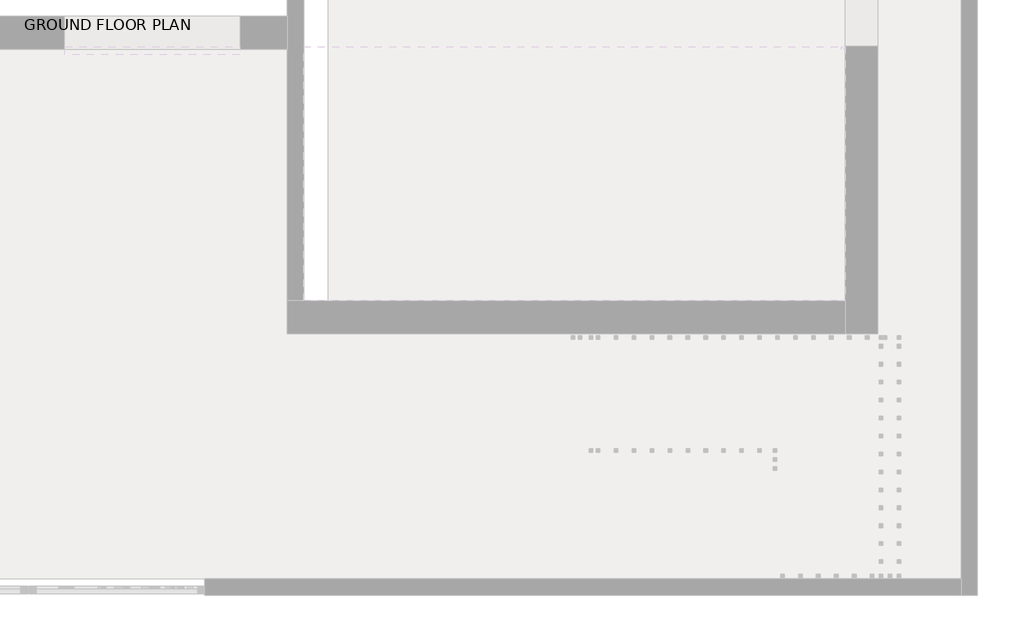
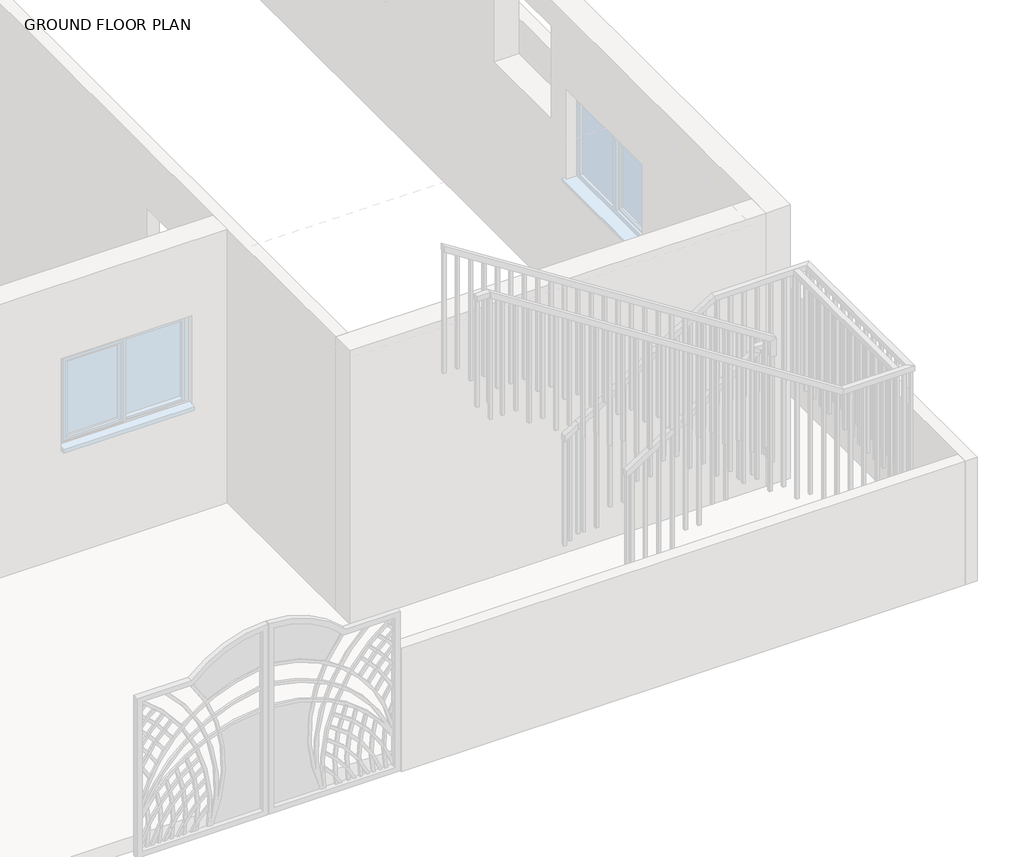
# One storey, part 20 of 23: 2 railings.
"""IFC4 building model written with IfcOpenShell, lengths in millimetres."""

from ifc_helpers import new_model, si_unit, frame, origin, place, context, project, spatial, polyline, outline, extrude, faceted_brep, element, save

model = new_model("IFC4")

# Units and contexts
model_context = context("Model", 3, world=origin())
ifc_project = project(units=[si_unit("LENGTHUNIT", "METRE", prefix="MILLI")], contexts=[model_context])

# Site, building, storey
site = spatial("IfcSite", under=ifc_project)
building = spatial("IfcBuilding", under=site)
storey = spatial("IfcBuildingStorey", under=building, Name="GROUND FLOOR PLAN", Elevation=487.68)

# Railings
placement = place(None, origin())
element("IfcRailing", 1, ObjectType="1100mm", at=placement, inside=storey, context=model_context, shape_type="SolidModel", body=[
    faceted_brep([(-8680.149573, -10220.0521308, 1912.8), (-8680.149573, -10220.0521308, 1853.4423995), (-8680.149573, -10270.0521308, 1853.4423995), (-8680.149573, -10270.0521308, 1912.8), (-7409.7306254, -10220.0521308, 2725.6), (-7395.1045513, -10220.0521308, 2675.6), (-7395.1045513, -10270.0521308, 2675.6), (-7409.7306254, -10270.0521308, 2725.6), (-6495.8132565, -10220.0521308, 2725.6), (-6495.8132565, -10220.0521308, 2675.6), (-6545.8132565, -10270.0521308, 2675.6), (-6545.8132565, -10270.0521308, 2725.6), (-6495.8132565, -11933.6860066, 2725.6), (-6495.8132565, -11933.6860066, 2675.6), (-6545.8132565, -11883.6860066, 2675.6), (-6545.8132565, -11883.6860066, 2725.6), (-7155.718398, -11933.6860066, 2725.6), (-7170.3479429, -11933.6860066, 2675.6), (-7170.3479429, -11883.6860066, 2675.6), (-7155.718398, -11883.6860066, 2725.6), (-10457.8773536, -11933.6860066, 4838.88), (-10457.8773536, -11883.6860066, 4838.88), (-10457.8773536, -11883.6860066, 4779.517542), (-10457.8773536, -11933.6860066, 4779.517542)], [[[0, 1, 2, 3]], [[1, 0, 4, 5]], [[2, 1, 5, 6]], [[3, 2, 6, 7]], [[0, 3, 7, 4]], [[5, 4, 8, 9]], [[6, 5, 9, 10]], [[7, 6, 10, 11]], [[4, 7, 11, 8]], [[9, 8, 12, 13]], [[10, 9, 13, 14]], [[11, 10, 14, 15]], [[8, 11, 15, 12]], [[13, 12, 16, 17]], [[14, 13, 17, 18]], [[15, 14, 18, 19]], [[12, 15, 19, 16]], [[20, 21, 22, 23]], [[17, 16, 20, 23]], [[18, 17, 23, 22]], [[19, 18, 22, 21]], [[16, 19, 21, 20]]]),
    extrude(outline(polyline([(4691.8007425, -10320.8132565), (4707.7999723, -10345.8132565), (3576.32, -10345.8132565), (3576.32, -10320.8132565), (4691.8007425, -10320.8132565)])), frame((0.0, -11921.1860066, 0.0), z_axis=(0.0, 1.0, 0.0), x_axis=(0.0, 0.0, 1.0)), (0.0, 0.0, 1.0), 25.0),
    extrude(outline(polyline([(4611.8045935, -10195.8132565), (4627.8038233, -10220.8132565), (3576.32, -10220.8132565), (3576.32, -10195.8132565), (4611.8045935, -10195.8132565)])), frame((0.0, -11921.1860066, 0.0), z_axis=(0.0, 1.0, 0.0), x_axis=(0.0, 0.0, 1.0)), (0.0, 0.0, 1.0), 25.0),
    extrude(outline(polyline([(4531.8084444, -10070.8132565), (4547.8076742, -10095.8132565), (3413.76, -10095.8132565), (3413.76, -10070.8132565), (4531.8084444, -10070.8132565)])), frame((0.0, -11921.1860066, 0.0), z_axis=(0.0, 1.0, 0.0), x_axis=(0.0, 0.0, 1.0)), (0.0, 0.0, 1.0), 25.0),
    extrude(outline(polyline([(4451.8122954, -9945.8132565), (4467.8115252, -9970.8132565), (3413.76, -9970.8132565), (3413.76, -9945.8132565), (4451.8122954, -9945.8132565)])), frame((0.0, -11921.1860066, 0.0), z_axis=(0.0, 1.0, 0.0), x_axis=(0.0, 0.0, 1.0)), (0.0, 0.0, 1.0), 25.0),
    extrude(outline(polyline([(4371.8161463, -9820.8132565), (4387.8153761, -9845.8132565), (3251.2, -9845.8132565), (3251.2, -9820.8132565), (4371.8161463, -9820.8132565)])), frame((0.0, -11921.1860066, 0.0), z_axis=(0.0, 1.0, 0.0), x_axis=(0.0, 0.0, 1.0)), (0.0, 0.0, 1.0), 25.0),
    extrude(outline(polyline([(4291.8423995, -9695.8132565), (4307.8371231, -9720.8132565), (3251.2, -9720.8132565), (3251.2, -9695.8132565), (4291.8423995, -9695.8132565)])), frame((0.0, -11921.1860066, 0.0), z_axis=(0.0, 1.0, 0.0), x_axis=(0.0, 0.0, 1.0)), (0.0, 0.0, 1.0), 25.0),
    extrude(outline(polyline([(4211.8238482, -9570.8132565), (4227.823078, -9595.8132565), (3088.64, -9595.8132565), (3088.64, -9570.8132565), (4211.8238482, -9570.8132565)])), frame((0.0, -11921.1860066, 0.0), z_axis=(0.0, 1.0, 0.0), x_axis=(0.0, 0.0, 1.0)), (0.0, 0.0, 1.0), 25.0),
    extrude(outline(polyline([(4131.8276992, -9445.8132565), (4147.826929, -9470.8132565), (3088.64, -9470.8132565), (3088.64, -9445.8132565), (4131.8276992, -9445.8132565)])), frame((0.0, -11921.1860066, 0.0), z_axis=(0.0, 1.0, 0.0), x_axis=(0.0, 0.0, 1.0)), (0.0, 0.0, 1.0), 25.0),
    extrude(outline(polyline([(4051.8315501, -9320.8132565), (4067.8307799, -9345.8132565), (2926.08, -9345.8132565), (2926.08, -9320.8132565), (4051.8315501, -9320.8132565)])), frame((0.0, -11921.1860066, 0.0), z_axis=(0.0, 1.0, 0.0), x_axis=(0.0, 0.0, 1.0)), (0.0, 0.0, 1.0), 25.0),
    extrude(outline(polyline([(3971.835401, -9195.8132565), (3987.8346309, -9220.8132565), (2926.08, -9220.8132565), (2926.08, -9195.8132565), (3971.835401, -9195.8132565)])), frame((0.0, -11921.1860066, 0.0), z_axis=(0.0, 1.0, 0.0), x_axis=(0.0, 0.0, 1.0)), (0.0, 0.0, 1.0), 25.0),
    extrude(outline(polyline([(3891.839252, -9070.8132565), (3907.8384818, -9095.8132565), (2763.52, -9095.8132565), (2763.52, -9070.8132565), (3891.839252, -9070.8132565)])), frame((0.0, -11921.1860066, 0.0), z_axis=(0.0, 1.0, 0.0), x_axis=(0.0, 0.0, 1.0)), (0.0, 0.0, 1.0), 25.0),
    extrude(outline(polyline([(3811.8431029, -8945.8132565), (3827.8423328, -8970.8132565), (2763.52, -8970.8132565), (2763.52, -8945.8132565), (3811.8431029, -8945.8132565)])), frame((0.0, -11921.1860066, 0.0), z_axis=(0.0, 1.0, 0.0), x_axis=(0.0, 0.0, 1.0)), (0.0, 0.0, 1.0), 25.0),
    extrude(outline(polyline([(3731.8469539, -8820.8132565), (3747.8461837, -8845.8132565), (2600.96, -8845.8132565), (2600.96, -8820.8132565), (3731.8469539, -8820.8132565)])), frame((0.0, -11921.1860066, 0.0), z_axis=(0.0, 1.0, 0.0), x_axis=(0.0, 0.0, 1.0)), (0.0, 0.0, 1.0), 25.0),
    extrude(outline(polyline([(3651.8508048, -8695.8132565), (3667.8500347, -8720.8132565), (2600.96, -8720.8132565), (2600.96, -8695.8132565), (3651.8508048, -8695.8132565)])), frame((0.0, -11921.1860066, 0.0), z_axis=(0.0, 1.0, 0.0), x_axis=(0.0, 0.0, 1.0)), (0.0, 0.0, 1.0), 25.0),
    extrude(outline(polyline([(3571.8546558, -8570.8132565), (3587.8538856, -8595.8132565), (2438.4, -8595.8132565), (2438.4, -8570.8132565), (3571.8546558, -8570.8132565)])), frame((0.0, -11921.1860066, 0.0), z_axis=(0.0, 1.0, 0.0), x_axis=(0.0, 0.0, 1.0)), (0.0, 0.0, 1.0), 25.0),
    extrude(outline(polyline([(3491.8585067, -8445.8132565), (3507.8577365, -8470.8132565), (2438.4, -8470.8132565), (2438.4, -8445.8132565), (3491.8585067, -8445.8132565)])), frame((0.0, -11921.1860066, 0.0), z_axis=(0.0, 1.0, 0.0), x_axis=(0.0, 0.0, 1.0)), (0.0, 0.0, 1.0), 25.0),
    extrude(outline(polyline([(3411.8623577, -8320.8132565), (3427.8615875, -8345.8132565), (2275.84, -8345.8132565), (2275.84, -8320.8132565), (3411.8623577, -8320.8132565)])), frame((0.0, -11921.1860066, 0.0), z_axis=(0.0, 1.0, 0.0), x_axis=(0.0, 0.0, 1.0)), (0.0, 0.0, 1.0), 25.0),
    extrude(outline(polyline([(3331.8662086, -8195.8132565), (3347.8654384, -8220.8132565), (2275.84, -8220.8132565), (2275.84, -8195.8132565), (3331.8662086, -8195.8132565)])), frame((0.0, -11921.1860066, 0.0), z_axis=(0.0, 1.0, 0.0), x_axis=(0.0, 0.0, 1.0)), (0.0, 0.0, 1.0), 25.0),
    extrude(outline(polyline([(3251.8700596, -8070.8132565), (3267.8692894, -8095.8132565), (2113.28, -8095.8132565), (2113.28, -8070.8132565), (3251.8700596, -8070.8132565)])), frame((0.0, -11921.1860066, 0.0), z_axis=(0.0, 1.0, 0.0), x_axis=(0.0, 0.0, 1.0)), (0.0, 0.0, 1.0), 25.0),
    extrude(outline(polyline([(3171.8739105, -7945.8132565), (3187.8731403, -7970.8132565), (2113.28, -7970.8132565), (2113.28, -7945.8132565), (3171.8739105, -7945.8132565)])), frame((0.0, -11921.1860066, 0.0), z_axis=(0.0, 1.0, 0.0), x_axis=(0.0, 0.0, 1.0)), (0.0, 0.0, 1.0), 25.0),
    extrude(outline(polyline([(3091.8777615, -7820.8132565), (3107.8769913, -7845.8132565), (1950.72, -7845.8132565), (1950.72, -7820.8132565), (3091.8777615, -7820.8132565)])), frame((0.0, -11921.1860066, 0.0), z_axis=(0.0, 1.0, 0.0), x_axis=(0.0, 0.0, 1.0)), (0.0, 0.0, 1.0), 25.0),
    extrude(outline(polyline([(3011.8816124, -7695.8132565), (3027.8808422, -7720.8132565), (1950.72, -7720.8132565), (1950.72, -7695.8132565), (3011.8816124, -7695.8132565)])), frame((0.0, -11921.1860066, 0.0), z_axis=(0.0, 1.0, 0.0), x_axis=(0.0, 0.0, 1.0)), (0.0, 0.0, 1.0), 25.0),
    extrude(outline(polyline([(2931.8854634, -7570.8132565), (2947.8846932, -7595.8132565), (1788.16, -7595.8132565), (1788.16, -7570.8132565), (2931.8854634, -7570.8132565)])), frame((0.0, -11921.1860066, 0.0), z_axis=(0.0, 1.0, 0.0), x_axis=(0.0, 0.0, 1.0)), (0.0, 0.0, 1.0), 25.0),
    extrude(outline(polyline([(2851.8893143, -7445.8132565), (2867.8885441, -7470.8132565), (1788.16, -7470.8132565), (1788.16, -7445.8132565), (2851.8893143, -7445.8132565)])), frame((0.0, -11921.1860066, 0.0), z_axis=(0.0, 1.0, 0.0), x_axis=(0.0, 0.0, 1.0)), (0.0, 0.0, 1.0), 25.0),
    extrude(outline(polyline([(2771.8931653, -7320.8132565), (2787.8923951, -7345.8132565), (1625.6, -7345.8132565), (1625.6, -7320.8132565), (2771.8931653, -7320.8132565)])), frame((0.0, -11921.1860066, 0.0), z_axis=(0.0, 1.0, 0.0), x_axis=(0.0, 0.0, 1.0)), (0.0, 0.0, 1.0), 25.0),
    extrude(outline(polyline([(2691.8970162, -7195.8132565), (2707.896246, -7220.8132565), (1625.6, -7220.8132565), (1625.6, -7195.8132565), (2691.8970162, -7195.8132565)])), frame((0.0, -11921.1860066, 0.0), z_axis=(0.0, 1.0, 0.0), x_axis=(0.0, 0.0, 1.0)), (0.0, 0.0, 1.0), 25.0),
    extrude(outline(polyline([(-7070.8132565, -11921.1860066), (-7095.8132565, -11921.1860066), (-7095.8132565, -11896.1860066), (-7070.8132565, -11896.1860066), (-7070.8132565, -11921.1860066)])), frame((0.0, 0.0, 1625.6), z_axis=(0.0, 0.0, 1.0), x_axis=(1.0, 0.0, 0.0)), (0.0, 0.0, 1.0), 1050.0),
    extrude(outline(polyline([(-6945.8132565, -11921.1860066), (-6970.8132565, -11921.1860066), (-6970.8132565, -11896.1860066), (-6945.8132565, -11896.1860066), (-6945.8132565, -11921.1860066)])), frame((0.0, 0.0, 1625.6), z_axis=(0.0, 0.0, 1.0), x_axis=(1.0, 0.0, 0.0)), (0.0, 0.0, 1.0), 1050.0),
    extrude(outline(polyline([(-6820.8132565, -11921.1860066), (-6845.8132565, -11921.1860066), (-6845.8132565, -11896.1860066), (-6820.8132565, -11896.1860066), (-6820.8132565, -11921.1860066)])), frame((0.0, 0.0, 1625.6), z_axis=(0.0, 0.0, 1.0), x_axis=(1.0, 0.0, 0.0)), (0.0, 0.0, 1.0), 1050.0),
    extrude(outline(polyline([(-6695.8132565, -11921.1860066), (-6720.8132565, -11921.1860066), (-6720.8132565, -11896.1860066), (-6695.8132565, -11896.1860066), (-6695.8132565, -11921.1860066)])), frame((0.0, 0.0, 1625.6), z_axis=(0.0, 0.0, 1.0), x_axis=(1.0, 0.0, 0.0)), (0.0, 0.0, 1.0), 1050.0),
    extrude(outline(polyline([(-6570.8132565, -11921.1860066), (-6595.8132565, -11921.1860066), (-6595.8132565, -11896.1860066), (-6570.8132565, -11896.1860066), (-6570.8132565, -11921.1860066)])), frame((0.0, 0.0, 1625.6), z_axis=(0.0, 0.0, 1.0), x_axis=(1.0, 0.0, 0.0)), (0.0, 0.0, 1.0), 1050.0),
    extrude(outline(polyline([(-6508.3132565, -11795.0521308), (-6508.3132565, -11820.0521308), (-6533.3132565, -11820.0521308), (-6533.3132565, -11795.0521308), (-6508.3132565, -11795.0521308)])), frame((0.0, 0.0, 1625.6), z_axis=(0.0, 0.0, 1.0), x_axis=(1.0, 0.0, 0.0)), (0.0, 0.0, 1.0), 1050.0),
    extrude(outline(polyline([(-6508.3132565, -11670.0521308), (-6508.3132565, -11695.0521308), (-6533.3132565, -11695.0521308), (-6533.3132565, -11670.0521308), (-6508.3132565, -11670.0521308)])), frame((0.0, 0.0, 1625.6), z_axis=(0.0, 0.0, 1.0), x_axis=(1.0, 0.0, 0.0)), (0.0, 0.0, 1.0), 1050.0),
    extrude(outline(polyline([(-6508.3132565, -11545.0521308), (-6508.3132565, -11570.0521308), (-6533.3132565, -11570.0521308), (-6533.3132565, -11545.0521308), (-6508.3132565, -11545.0521308)])), frame((0.0, 0.0, 1625.6), z_axis=(0.0, 0.0, 1.0), x_axis=(1.0, 0.0, 0.0)), (0.0, 0.0, 1.0), 1050.0),
    extrude(outline(polyline([(-6508.3132565, -11420.0521308), (-6508.3132565, -11445.0521308), (-6533.3132565, -11445.0521308), (-6533.3132565, -11420.0521308), (-6508.3132565, -11420.0521308)])), frame((0.0, 0.0, 1625.6), z_axis=(0.0, 0.0, 1.0), x_axis=(1.0, 0.0, 0.0)), (0.0, 0.0, 1.0), 1050.0),
    extrude(outline(polyline([(-6508.3132565, -11295.0521308), (-6508.3132565, -11320.0521308), (-6533.3132565, -11320.0521308), (-6533.3132565, -11295.0521308), (-6508.3132565, -11295.0521308)])), frame((0.0, 0.0, 1625.6), z_axis=(0.0, 0.0, 1.0), x_axis=(1.0, 0.0, 0.0)), (0.0, 0.0, 1.0), 1050.0),
    extrude(outline(polyline([(-6508.3132565, -11170.0521308), (-6508.3132565, -11195.0521308), (-6533.3132565, -11195.0521308), (-6533.3132565, -11170.0521308), (-6508.3132565, -11170.0521308)])), frame((0.0, 0.0, 1625.6), z_axis=(0.0, 0.0, 1.0), x_axis=(1.0, 0.0, 0.0)), (0.0, 0.0, 1.0), 1050.0),
    extrude(outline(polyline([(-6508.3132565, -11045.0521308), (-6508.3132565, -11070.0521308), (-6533.3132565, -11070.0521308), (-6533.3132565, -11045.0521308), (-6508.3132565, -11045.0521308)])), frame((0.0, 0.0, 1625.6), z_axis=(0.0, 0.0, 1.0), x_axis=(1.0, 0.0, 0.0)), (0.0, 0.0, 1.0), 1050.0),
    extrude(outline(polyline([(-6508.3132565, -10920.0521308), (-6508.3132565, -10945.0521308), (-6533.3132565, -10945.0521308), (-6533.3132565, -10920.0521308), (-6508.3132565, -10920.0521308)])), frame((0.0, 0.0, 1625.6), z_axis=(0.0, 0.0, 1.0), x_axis=(1.0, 0.0, 0.0)), (0.0, 0.0, 1.0), 1050.0),
    extrude(outline(polyline([(-6508.3132565, -10795.0521308), (-6508.3132565, -10820.0521308), (-6533.3132565, -10820.0521308), (-6533.3132565, -10795.0521308), (-6508.3132565, -10795.0521308)])), frame((0.0, 0.0, 1625.6), z_axis=(0.0, 0.0, 1.0), x_axis=(1.0, 0.0, 0.0)), (0.0, 0.0, 1.0), 1050.0),
    extrude(outline(polyline([(-6508.3132565, -10670.0521308), (-6508.3132565, -10695.0521308), (-6533.3132565, -10695.0521308), (-6533.3132565, -10670.0521308), (-6508.3132565, -10670.0521308)])), frame((0.0, 0.0, 1625.6), z_axis=(0.0, 0.0, 1.0), x_axis=(1.0, 0.0, 0.0)), (0.0, 0.0, 1.0), 1050.0),
    extrude(outline(polyline([(-6508.3132565, -10545.0521308), (-6508.3132565, -10570.0521308), (-6533.3132565, -10570.0521308), (-6533.3132565, -10545.0521308), (-6508.3132565, -10545.0521308)])), frame((0.0, 0.0, 1625.6), z_axis=(0.0, 0.0, 1.0), x_axis=(1.0, 0.0, 0.0)), (0.0, 0.0, 1.0), 1050.0),
    extrude(outline(polyline([(-6508.3132565, -10420.0521308), (-6508.3132565, -10445.0521308), (-6533.3132565, -10445.0521308), (-6533.3132565, -10420.0521308), (-6508.3132565, -10420.0521308)])), frame((0.0, 0.0, 1625.6), z_axis=(0.0, 0.0, 1.0), x_axis=(1.0, 0.0, 0.0)), (0.0, 0.0, 1.0), 1050.0),
    extrude(outline(polyline([(-6508.3132565, -10295.0521308), (-6508.3132565, -10320.0521308), (-6533.3132565, -10320.0521308), (-6533.3132565, -10295.0521308), (-6508.3132565, -10295.0521308)])), frame((0.0, 0.0, 1625.6), z_axis=(0.0, 0.0, 1.0), x_axis=(1.0, 0.0, 0.0)), (0.0, 0.0, 1.0), 1050.0),
    extrude(outline(polyline([(-6630.149573, -10232.5521308), (-6605.149573, -10232.5521308), (-6605.149573, -10257.5521308), (-6630.149573, -10257.5521308), (-6630.149573, -10232.5521308)])), frame((0.0, 0.0, 1625.6), z_axis=(0.0, 0.0, 1.0), x_axis=(1.0, 0.0, 0.0)), (0.0, 0.0, 1.0), 1050.0),
    extrude(outline(polyline([(-6755.149573, -10232.5521308), (-6730.149573, -10232.5521308), (-6730.149573, -10257.5521308), (-6755.149573, -10257.5521308), (-6755.149573, -10232.5521308)])), frame((0.0, 0.0, 1625.6), z_axis=(0.0, 0.0, 1.0), x_axis=(1.0, 0.0, 0.0)), (0.0, 0.0, 1.0), 1050.0),
    extrude(outline(polyline([(-6880.149573, -10232.5521308), (-6855.149573, -10232.5521308), (-6855.149573, -10257.5521308), (-6880.149573, -10257.5521308), (-6880.149573, -10232.5521308)])), frame((0.0, 0.0, 1625.6), z_axis=(0.0, 0.0, 1.0), x_axis=(1.0, 0.0, 0.0)), (0.0, 0.0, 1.0), 1050.0),
    extrude(outline(polyline([(-7005.149573, -10232.5521308), (-6980.149573, -10232.5521308), (-6980.149573, -10257.5521308), (-7005.149573, -10257.5521308), (-7005.149573, -10232.5521308)])), frame((0.0, 0.0, 1625.6), z_axis=(0.0, 0.0, 1.0), x_axis=(1.0, 0.0, 0.0)), (0.0, 0.0, 1.0), 1050.0),
    extrude(outline(polyline([(-7130.149573, -10232.5521308), (-7105.149573, -10232.5521308), (-7105.149573, -10257.5521308), (-7130.149573, -10257.5521308), (-7130.149573, -10232.5521308)])), frame((0.0, 0.0, 1625.6), z_axis=(0.0, 0.0, 1.0), x_axis=(1.0, 0.0, 0.0)), (0.0, 0.0, 1.0), 1050.0),
    extrude(outline(polyline([(-7255.149573, -10232.5521308), (-7230.149573, -10232.5521308), (-7230.149573, -10257.5521308), (-7255.149573, -10257.5521308), (-7255.149573, -10232.5521308)])), frame((0.0, 0.0, 1625.6), z_axis=(0.0, 0.0, 1.0), x_axis=(1.0, 0.0, 0.0)), (0.0, 0.0, 1.0), 1050.0),
    extrude(outline(polyline([(-7380.149573, -10232.5521308), (-7355.149573, -10232.5521308), (-7355.149573, -10257.5521308), (-7380.149573, -10257.5521308), (-7380.149573, -10232.5521308)])), frame((0.0, 0.0, 1625.6), z_axis=(0.0, 0.0, 1.0), x_axis=(1.0, 0.0, 0.0)), (0.0, 0.0, 1.0), 1050.0),
    extrude(outline(polyline([(1463.04, -7505.149573), (1463.04, -7480.149573), (2621.1891352, -7480.149573), (2605.1944115, -7505.149573), (1463.04, -7505.149573)])), frame((0.0, -10257.5521308, 0.0), z_axis=(0.0, 1.0, 0.0), x_axis=(0.0, 0.0, 1.0)), (0.0, 0.0, 1.0), 25.0),
    extrude(outline(polyline([(1463.04, -7630.149573), (1463.04, -7605.149573), (2541.2155169, -7605.149573), (2525.2207932, -7630.149573), (1463.04, -7630.149573)])), frame((0.0, -10257.5521308, 0.0), z_axis=(0.0, 1.0, 0.0), x_axis=(0.0, 0.0, 1.0)), (0.0, 0.0, 1.0), 25.0),
    extrude(outline(polyline([(1300.48, -7755.149573), (1300.48, -7730.149573), (2461.2418986, -7730.149573), (2445.2471749, -7755.149573), (1300.48, -7755.149573)])), frame((0.0, -10257.5521308, 0.0), z_axis=(0.0, 1.0, 0.0), x_axis=(0.0, 0.0, 1.0)), (0.0, 0.0, 1.0), 25.0),
    extrude(outline(polyline([(1300.48, -7880.149573), (1300.48, -7855.149573), (2381.2682803, -7855.149573), (2365.2735566, -7880.149573), (1300.48, -7880.149573)])), frame((0.0, -10257.5521308, 0.0), z_axis=(0.0, 1.0, 0.0), x_axis=(0.0, 0.0, 1.0)), (0.0, 0.0, 1.0), 25.0),
    extrude(outline(polyline([(1137.92, -8005.149573), (1137.92, -7980.149573), (2301.294662, -7980.149573), (2285.2999383, -8005.149573), (1137.92, -8005.149573)])), frame((0.0, -10257.5521308, 0.0), z_axis=(0.0, 1.0, 0.0), x_axis=(0.0, 0.0, 1.0)), (0.0, 0.0, 1.0), 25.0),
    extrude(outline(polyline([(1137.92, -8130.149573), (1137.92, -8105.149573), (2221.3210437, -8105.149573), (2205.32632, -8130.149573), (1137.92, -8130.149573)])), frame((0.0, -10257.5521308, 0.0), z_axis=(0.0, 1.0, 0.0), x_axis=(0.0, 0.0, 1.0)), (0.0, 0.0, 1.0), 25.0),
    extrude(outline(polyline([(975.36, -8255.149573), (975.36, -8230.149573), (2141.3474254, -8230.149573), (2125.3527017, -8255.149573), (975.36, -8255.149573)])), frame((0.0, -10257.5521308, 0.0), z_axis=(0.0, 1.0, 0.0), x_axis=(0.0, 0.0, 1.0)), (0.0, 0.0, 1.0), 25.0),
    extrude(outline(polyline([(975.36, -8380.149573), (975.36, -8355.149573), (2061.3738071, -8355.149573), (2045.3790834, -8380.149573), (975.36, -8380.149573)])), frame((0.0, -10257.5521308, 0.0), z_axis=(0.0, 1.0, 0.0), x_axis=(0.0, 0.0, 1.0)), (0.0, 0.0, 1.0), 25.0),
    extrude(outline(polyline([(812.8, -8505.149573), (812.8, -8480.149573), (1981.4001888, -8480.149573), (1965.4054651, -8505.149573), (812.8, -8505.149573)])), frame((0.0, -10257.5521308, 0.0), z_axis=(0.0, 1.0, 0.0), x_axis=(0.0, 0.0, 1.0)), (0.0, 0.0, 1.0), 25.0),
    extrude(outline(polyline([(812.8, -8630.149573), (812.8, -8605.149573), (1901.4265705, -8605.149573), (1885.4318468, -8630.149573), (812.8, -8630.149573)])), frame((0.0, -10257.5521308, 0.0), z_axis=(0.0, 1.0, 0.0), x_axis=(0.0, 0.0, 1.0)), (0.0, 0.0, 1.0), 25.0),
    extrude(outline(polyline([(-6508.3132565, -11896.1860066), (-6508.3132565, -11921.1860066), (-6533.3132565, -11921.1860066), (-6533.3132565, -11896.1860066), (-6508.3132565, -11896.1860066)])), frame((0.0, 0.0, 1625.6), z_axis=(0.0, 0.0, 1.0), x_axis=(1.0, 0.0, 0.0)), (0.0, 0.0, 1.0), 1050.0),
    extrude(outline(polyline([(-6533.3132565, -10232.5521308), (-6508.3132565, -10232.5521308), (-6508.3132565, -10257.5521308), (-6533.3132565, -10257.5521308), (-6533.3132565, -10232.5521308)])), frame((0.0, 0.0, 1625.6), z_axis=(0.0, 0.0, 1.0), x_axis=(1.0, 0.0, 0.0)), (0.0, 0.0, 1.0), 1050.0),
    extrude(outline(polyline([(4763.5183122, -10432.8773536), (4779.517542, -10457.8773536), (3576.32, -10457.8773536), (3576.32, -10432.8773536), (4763.5183122, -10432.8773536)])), frame((0.0, -11921.1860066, 0.0), z_axis=(0.0, 1.0, 0.0), x_axis=(0.0, 0.0, 1.0)), (0.0, 0.0, 1.0), 25.0),
    extrude(outline(polyline([(812.8, -8680.149573), (812.8, -8655.149573), (1869.4371231, -8655.149573), (1853.4423995, -8680.149573), (812.8, -8680.149573)])), frame((0.0, -10257.5521308, 0.0), z_axis=(0.0, 1.0, 0.0), x_axis=(0.0, 0.0, 1.0)), (0.0, 0.0, 1.0), 25.0),
])
element("IfcRailing", 2, ObjectType="1100mm", at=placement, inside=storey, context=model_context, shape_type="SolidModel", body=[
    faceted_brep([(-8680.149573, -11007.9255223, 1912.8), (-8680.149573, -11007.9255223, 1853.4423995), (-8680.149573, -11057.9255223, 1853.4423995), (-8680.149573, -11057.9255223, 1912.8), (-7484.3306254, -11007.9255223, 2677.8717446), (-7434.3306254, -11007.9255223, 2650.5035914), (-7434.3306254, -11057.9255223, 2650.5035914), (-7484.3306254, -11057.9255223, 2677.8717446), (-7484.3306254, -11007.9255223, 2725.6), (-7434.3306254, -11007.9255223, 2675.6), (-7434.3306254, -11057.9255223, 2675.6), (-7484.3306254, -11057.9255223, 2725.6), (-7359.3306254, -11007.9255223, 2725.6), (-7359.3306254, -11007.9255223, 2675.6), (-7409.3306254, -11057.9255223, 2675.6), (-7409.3306254, -11057.9255223, 2725.6), (-7359.3306254, -11132.9255223, 2725.6), (-7359.3306254, -11132.9255223, 2675.6), (-7409.3306254, -11132.9255223, 2675.6), (-7409.3306254, -11132.9255223, 2725.6), (-7359.3306254, -11134.9255223, 2725.6), (-7409.3306254, -11134.9255223, 2725.6), (-7409.3306254, -11184.9255223, 2675.6), (-7359.3306254, -11184.9255223, 2675.6)], [[[0, 1, 2, 3]], [[1, 0, 4, 5]], [[2, 1, 5, 6]], [[3, 2, 6, 7]], [[0, 3, 7, 4]], [[5, 4, 8, 9]], [[6, 5, 9, 10]], [[7, 6, 10, 11]], [[4, 7, 11, 8]], [[9, 8, 12, 13]], [[10, 9, 13, 14]], [[11, 10, 14, 15]], [[8, 11, 15, 12]], [[13, 12, 16, 17]], [[14, 13, 17, 18]], [[15, 14, 18, 19]], [[12, 15, 19, 16]], [[20, 21, 22, 23]], [[17, 16, 20, 23]], [[18, 17, 23, 22]], [[19, 18, 22, 21]], [[16, 19, 21, 20]]]),
    faceted_brep([(-7359.3306254, -11184.9255223, 2855.9055527), (-7409.3306254, -11184.9255223, 2828.5415543), (-7409.3306254, -11134.9255223, 2828.5415543), (-7359.3306254, -11134.9255223, 2855.9055527), (-10457.8773536, -11184.9255223, 4838.88), (-10457.8773536, -11134.9255223, 4838.88), (-10457.8773536, -11134.9255223, 4779.517542), (-10457.8773536, -11184.9255223, 4779.517542)], [[[0, 1, 2, 3]], [[4, 5, 6, 7]], [[1, 0, 4, 7]], [[2, 1, 7, 6]], [[3, 2, 6, 5]], [[0, 3, 5, 4]]]),
    faceted_brep([(-7359.3306254, -11134.9255223, 2725.6), (-7359.3306254, -11184.9255223, 2675.6), (-7409.3306254, -11184.9255223, 2675.6), (-7409.3306254, -11134.9255223, 2725.6), (-7359.3306254, -11134.9255223, 2855.9055527), (-7409.3306254, -11134.9255223, 2828.5415543), (-7409.3306254, -11184.9255223, 2828.5415543), (-7359.3306254, -11184.9255223, 2855.9055527)], [[[0, 1, 2, 3]], [[4, 5, 6, 7]], [[1, 0, 4, 7]], [[2, 1, 7, 6]], [[3, 2, 6, 5]], [[0, 3, 5, 4]]]),
    extrude(outline(polyline([(3576.32, -10434.3306254), (4764.4483614, -10434.3306254), (4780.4475912, -10459.3306254), (3576.32, -10459.3306254), (3576.32, -10434.3306254)])), frame((0.0, -11172.4255223, 0.0), z_axis=(0.0, 1.0, 0.0), x_axis=(0.0, 0.0, 1.0)), (0.0, 0.0, 1.0), 25.0),
    extrude(outline(polyline([(3576.32, -10309.3306254), (4684.4522123, -10309.3306254), (4700.4514422, -10334.3306254), (3576.32, -10334.3306254), (3576.32, -10309.3306254)])), frame((0.0, -11172.4255223, 0.0), z_axis=(0.0, 1.0, 0.0), x_axis=(0.0, 0.0, 1.0)), (0.0, 0.0, 1.0), 25.0),
    extrude(outline(polyline([(3413.76, -10184.3306254), (4604.4560633, -10184.3306254), (4620.4552931, -10209.3306254), (3413.76, -10209.3306254), (3413.76, -10184.3306254)])), frame((0.0, -11172.4255223, 0.0), z_axis=(0.0, 1.0, 0.0), x_axis=(0.0, 0.0, 1.0)), (0.0, 0.0, 1.0), 25.0),
    extrude(outline(polyline([(3413.76, -10059.3306254), (4524.4599142, -10059.3306254), (4540.459144, -10084.3306254), (3413.76, -10084.3306254), (3413.76, -10059.3306254)])), frame((0.0, -11172.4255223, 0.0), z_axis=(0.0, 1.0, 0.0), x_axis=(0.0, 0.0, 1.0)), (0.0, 0.0, 1.0), 25.0),
    extrude(outline(polyline([(3251.2, -9934.3306254), (4444.4637652, -9934.3306254), (4460.462995, -9959.3306254), (3251.2, -9959.3306254), (3251.2, -9934.3306254)])), frame((0.0, -11172.4255223, 0.0), z_axis=(0.0, 1.0, 0.0), x_axis=(0.0, 0.0, 1.0)), (0.0, 0.0, 1.0), 25.0),
    extrude(outline(polyline([(3251.2, -9809.3306254), (4364.4676161, -9809.3306254), (4380.4668459, -9834.3306254), (3251.2, -9834.3306254), (3251.2, -9809.3306254)])), frame((0.0, -11172.4255223, 0.0), z_axis=(0.0, 1.0, 0.0), x_axis=(0.0, 0.0, 1.0)), (0.0, 0.0, 1.0), 25.0),
    extrude(outline(polyline([(3251.2, -9684.3306254), (4284.4714671, -9684.3306254), (4300.4706969, -9709.3306254), (3251.2, -9709.3306254), (3251.2, -9684.3306254)])), frame((0.0, -11172.4255223, 0.0), z_axis=(0.0, 1.0, 0.0), x_axis=(0.0, 0.0, 1.0)), (0.0, 0.0, 1.0), 25.0),
    extrude(outline(polyline([(3088.64, -9559.3306254), (4204.475318, -9559.3306254), (4220.4745478, -9584.3306254), (3088.64, -9584.3306254), (3088.64, -9559.3306254)])), frame((0.0, -11172.4255223, 0.0), z_axis=(0.0, 1.0, 0.0), x_axis=(0.0, 0.0, 1.0)), (0.0, 0.0, 1.0), 25.0),
    extrude(outline(polyline([(3088.64, -9434.3306254), (4124.479169, -9434.3306254), (4140.4783988, -9459.3306254), (3088.64, -9459.3306254), (3088.64, -9434.3306254)])), frame((0.0, -11172.4255223, 0.0), z_axis=(0.0, 1.0, 0.0), x_axis=(0.0, 0.0, 1.0)), (0.0, 0.0, 1.0), 25.0),
    extrude(outline(polyline([(2926.08, -9309.3306254), (4044.4830199, -9309.3306254), (4060.4822497, -9334.3306254), (2926.08, -9334.3306254), (2926.08, -9309.3306254)])), frame((0.0, -11172.4255223, 0.0), z_axis=(0.0, 1.0, 0.0), x_axis=(0.0, 0.0, 1.0)), (0.0, 0.0, 1.0), 25.0),
    extrude(outline(polyline([(2926.08, -9184.3306254), (3964.4868709, -9184.3306254), (3980.4861007, -9209.3306254), (2926.08, -9209.3306254), (2926.08, -9184.3306254)])), frame((0.0, -11172.4255223, 0.0), z_axis=(0.0, 1.0, 0.0), x_axis=(0.0, 0.0, 1.0)), (0.0, 0.0, 1.0), 25.0),
    extrude(outline(polyline([(2763.52, -9059.3306254), (3884.4907218, -9059.3306254), (3900.4899516, -9084.3306254), (2763.52, -9084.3306254), (2763.52, -9059.3306254)])), frame((0.0, -11172.4255223, 0.0), z_axis=(0.0, 1.0, 0.0), x_axis=(0.0, 0.0, 1.0)), (0.0, 0.0, 1.0), 25.0),
    extrude(outline(polyline([(2763.52, -8934.3306254), (3804.4945728, -8934.3306254), (3820.4938026, -8959.3306254), (2763.52, -8959.3306254), (2763.52, -8934.3306254)])), frame((0.0, -11172.4255223, 0.0), z_axis=(0.0, 1.0, 0.0), x_axis=(0.0, 0.0, 1.0)), (0.0, 0.0, 1.0), 25.0),
    extrude(outline(polyline([(2600.96, -8809.3306254), (3724.4984237, -8809.3306254), (3740.4976535, -8834.3306254), (2600.96, -8834.3306254), (2600.96, -8809.3306254)])), frame((0.0, -11172.4255223, 0.0), z_axis=(0.0, 1.0, 0.0), x_axis=(0.0, 0.0, 1.0)), (0.0, 0.0, 1.0), 25.0),
    extrude(outline(polyline([(2600.96, -8684.3306254), (3644.5022747, -8684.3306254), (3660.5015045, -8709.3306254), (2600.96, -8709.3306254), (2600.96, -8684.3306254)])), frame((0.0, -11172.4255223, 0.0), z_axis=(0.0, 1.0, 0.0), x_axis=(0.0, 0.0, 1.0)), (0.0, 0.0, 1.0), 25.0),
    extrude(outline(polyline([(2438.4, -8559.3306254), (3564.5061256, -8559.3306254), (3580.5053554, -8584.3306254), (2438.4, -8584.3306254), (2438.4, -8559.3306254)])), frame((0.0, -11172.4255223, 0.0), z_axis=(0.0, 1.0, 0.0), x_axis=(0.0, 0.0, 1.0)), (0.0, 0.0, 1.0), 25.0),
    extrude(outline(polyline([(2438.4, -8434.3306254), (3484.5099766, -8434.3306254), (3500.5092064, -8459.3306254), (2438.4, -8459.3306254), (2438.4, -8434.3306254)])), frame((0.0, -11172.4255223, 0.0), z_axis=(0.0, 1.0, 0.0), x_axis=(0.0, 0.0, 1.0)), (0.0, 0.0, 1.0), 25.0),
    extrude(outline(polyline([(2275.84, -8309.3306254), (3404.5138275, -8309.3306254), (3420.5130573, -8334.3306254), (2275.84, -8334.3306254), (2275.84, -8309.3306254)])), frame((0.0, -11172.4255223, 0.0), z_axis=(0.0, 1.0, 0.0), x_axis=(0.0, 0.0, 1.0)), (0.0, 0.0, 1.0), 25.0),
    extrude(outline(polyline([(2275.84, -8184.3306254), (3324.5176785, -8184.3306254), (3340.5169083, -8209.3306254), (2275.84, -8209.3306254), (2275.84, -8184.3306254)])), frame((0.0, -11172.4255223, 0.0), z_axis=(0.0, 1.0, 0.0), x_axis=(0.0, 0.0, 1.0)), (0.0, 0.0, 1.0), 25.0),
    extrude(outline(polyline([(2113.28, -8059.3306254), (3244.5215294, -8059.3306254), (3260.5207592, -8084.3306254), (2113.28, -8084.3306254), (2113.28, -8059.3306254)])), frame((0.0, -11172.4255223, 0.0), z_axis=(0.0, 1.0, 0.0), x_axis=(0.0, 0.0, 1.0)), (0.0, 0.0, 1.0), 25.0),
    extrude(outline(polyline([(2113.28, -7934.3306254), (3164.5253804, -7934.3306254), (3180.5246102, -7959.3306254), (2113.28, -7959.3306254), (2113.28, -7934.3306254)])), frame((0.0, -11172.4255223, 0.0), z_axis=(0.0, 1.0, 0.0), x_axis=(0.0, 0.0, 1.0)), (0.0, 0.0, 1.0), 25.0),
    extrude(outline(polyline([(1950.72, -7809.3306254), (3084.5292313, -7809.3306254), (3100.5284611, -7834.3306254), (1950.72, -7834.3306254), (1950.72, -7809.3306254)])), frame((0.0, -11172.4255223, 0.0), z_axis=(0.0, 1.0, 0.0), x_axis=(0.0, 0.0, 1.0)), (0.0, 0.0, 1.0), 25.0),
    extrude(outline(polyline([(1950.72, -7684.3306254), (3004.5330823, -7684.3306254), (3020.5323121, -7709.3306254), (1950.72, -7709.3306254), (1950.72, -7684.3306254)])), frame((0.0, -11172.4255223, 0.0), z_axis=(0.0, 1.0, 0.0), x_axis=(0.0, 0.0, 1.0)), (0.0, 0.0, 1.0), 25.0),
    extrude(outline(polyline([(1788.16, -7559.3306254), (2924.5369332, -7559.3306254), (2940.536163, -7584.3306254), (1788.16, -7584.3306254), (1788.16, -7559.3306254)])), frame((0.0, -11172.4255223, 0.0), z_axis=(0.0, 1.0, 0.0), x_axis=(0.0, 0.0, 1.0)), (0.0, 0.0, 1.0), 25.0),
    extrude(outline(polyline([(1788.16, -7434.3306254), (2844.5407841, -7434.3306254), (2860.540014, -7459.3306254), (1788.16, -7459.3306254), (1788.16, -7434.3306254)])), frame((0.0, -11172.4255223, 0.0), z_axis=(0.0, 1.0, 0.0), x_axis=(0.0, 0.0, 1.0)), (0.0, 0.0, 1.0), 25.0),
    extrude(outline(polyline([(-7396.8306254, -11082.9255223), (-7371.8306254, -11082.9255223), (-7371.8306254, -11107.9255223), (-7396.8306254, -11107.9255223), (-7396.8306254, -11082.9255223)])), frame((0.0, 0.0, 1625.6), z_axis=(0.0, 0.0, 1.0), x_axis=(1.0, 0.0, 0.0)), (0.0, 0.0, 1.0), 1050.0),
    extrude(outline(polyline([(2605.1944115, -7505.149573), (1463.04, -7505.149573), (1463.04, -7480.149573), (2621.1891352, -7480.149573), (2605.1944115, -7505.149573)])), frame((0.0, -11045.4255223, 0.0), z_axis=(0.0, 1.0, 0.0), x_axis=(0.0, 0.0, 1.0)), (0.0, 0.0, 1.0), 25.0),
    extrude(outline(polyline([(2525.2207932, -7630.149573), (1463.04, -7630.149573), (1463.04, -7605.149573), (2541.2155169, -7605.149573), (2525.2207932, -7630.149573)])), frame((0.0, -11045.4255223, 0.0), z_axis=(0.0, 1.0, 0.0), x_axis=(0.0, 0.0, 1.0)), (0.0, 0.0, 1.0), 25.0),
    extrude(outline(polyline([(2445.2471749, -7755.149573), (1300.48, -7755.149573), (1300.48, -7730.149573), (2461.2418986, -7730.149573), (2445.2471749, -7755.149573)])), frame((0.0, -11045.4255223, 0.0), z_axis=(0.0, 1.0, 0.0), x_axis=(0.0, 0.0, 1.0)), (0.0, 0.0, 1.0), 25.0),
    extrude(outline(polyline([(2365.2735566, -7880.149573), (1300.48, -7880.149573), (1300.48, -7855.149573), (2381.2682803, -7855.149573), (2365.2735566, -7880.149573)])), frame((0.0, -11045.4255223, 0.0), z_axis=(0.0, 1.0, 0.0), x_axis=(0.0, 0.0, 1.0)), (0.0, 0.0, 1.0), 25.0),
    extrude(outline(polyline([(2285.2999383, -8005.149573), (1137.92, -8005.149573), (1137.92, -7980.149573), (2301.294662, -7980.149573), (2285.2999383, -8005.149573)])), frame((0.0, -11045.4255223, 0.0), z_axis=(0.0, 1.0, 0.0), x_axis=(0.0, 0.0, 1.0)), (0.0, 0.0, 1.0), 25.0),
    extrude(outline(polyline([(2205.32632, -8130.149573), (1137.92, -8130.149573), (1137.92, -8105.149573), (2221.3210437, -8105.149573), (2205.32632, -8130.149573)])), frame((0.0, -11045.4255223, 0.0), z_axis=(0.0, 1.0, 0.0), x_axis=(0.0, 0.0, 1.0)), (0.0, 0.0, 1.0), 25.0),
    extrude(outline(polyline([(2125.3527017, -8255.149573), (975.36, -8255.149573), (975.36, -8230.149573), (2141.3474254, -8230.149573), (2125.3527017, -8255.149573)])), frame((0.0, -11045.4255223, 0.0), z_axis=(0.0, 1.0, 0.0), x_axis=(0.0, 0.0, 1.0)), (0.0, 0.0, 1.0), 25.0),
    extrude(outline(polyline([(2045.3790834, -8380.149573), (975.36, -8380.149573), (975.36, -8355.149573), (2061.3738071, -8355.149573), (2045.3790834, -8380.149573)])), frame((0.0, -11045.4255223, 0.0), z_axis=(0.0, 1.0, 0.0), x_axis=(0.0, 0.0, 1.0)), (0.0, 0.0, 1.0), 25.0),
    extrude(outline(polyline([(1965.4054651, -8505.149573), (812.8, -8505.149573), (812.8, -8480.149573), (1981.4001888, -8480.149573), (1965.4054651, -8505.149573)])), frame((0.0, -11045.4255223, 0.0), z_axis=(0.0, 1.0, 0.0), x_axis=(0.0, 0.0, 1.0)), (0.0, 0.0, 1.0), 25.0),
    extrude(outline(polyline([(1885.4318468, -8630.149573), (812.8, -8630.149573), (812.8, -8605.149573), (1901.4265705, -8605.149573), (1885.4318468, -8630.149573)])), frame((0.0, -11045.4255223, 0.0), z_axis=(0.0, 1.0, 0.0), x_axis=(0.0, 0.0, 1.0)), (0.0, 0.0, 1.0), 25.0),
    extrude(outline(polyline([(-7396.8306254, -11147.4255223), (-7371.8306254, -11147.4255223), (-7371.8306254, -11172.4255223), (-7396.8306254, -11172.4255223), (-7396.8306254, -11147.4255223)])), frame((0.0, 0.0, 1625.6), z_axis=(0.0, 0.0, 1.0), x_axis=(1.0, 0.0, 0.0)), (0.0, 0.0, 1.0), 1050.0),
    extrude(outline(polyline([(-7396.8306254, -11045.4255223), (-7396.8306254, -11020.4255223), (-7371.8306254, -11020.4255223), (-7371.8306254, -11045.4255223), (-7396.8306254, -11045.4255223)])), frame((0.0, 0.0, 1625.6), z_axis=(0.0, 0.0, 1.0), x_axis=(1.0, 0.0, 0.0)), (0.0, 0.0, 1.0), 1050.0),
    extrude(outline(polyline([(3576.32, -10432.8773536), (4763.5183122, -10432.8773536), (4779.517542, -10457.8773536), (3576.32, -10457.8773536), (3576.32, -10432.8773536)])), frame((0.0, -11172.4255223, 0.0), z_axis=(0.0, 1.0, 0.0), x_axis=(0.0, 0.0, 1.0)), (0.0, 0.0, 1.0), 25.0),
    extrude(outline(polyline([(1853.4423995, -8680.149573), (812.8, -8680.149573), (812.8, -8655.149573), (1869.4371231, -8655.149573), (1853.4423995, -8680.149573)])), frame((0.0, -11045.4255223, 0.0), z_axis=(0.0, 1.0, 0.0), x_axis=(0.0, 0.0, 1.0)), (0.0, 0.0, 1.0), 25.0),
])

save(model, "model.ifc")

# Revit data of these elements
# Type "1100mm"
#   built-in parameter 1008612 = 0.019685 (stored number, unit not read)
#   built-in parameter 1008611 = 0.019685 (stored number, unit not read)
#   built-in parameter 1008609 = 0.902231 (stored number, unit not read)
#   built-in parameter 1008604 = 0.19685 (stored number, unit not read)
#   built-in parameter 1008603 = 0.164042 (stored number, unit not read)
#   Railing Height = 3.608924 ft
#   built-in parameter 1008630 = 2
#   built-in parameter 1008610 = 2
#   built-in parameter 1008608 = 1
#   built-in parameter 1008618 = Baluster_Square : 25mm
# Elements 1, 2 (IfcRailing, "1100mm")
#   Phase Created = New Construction
